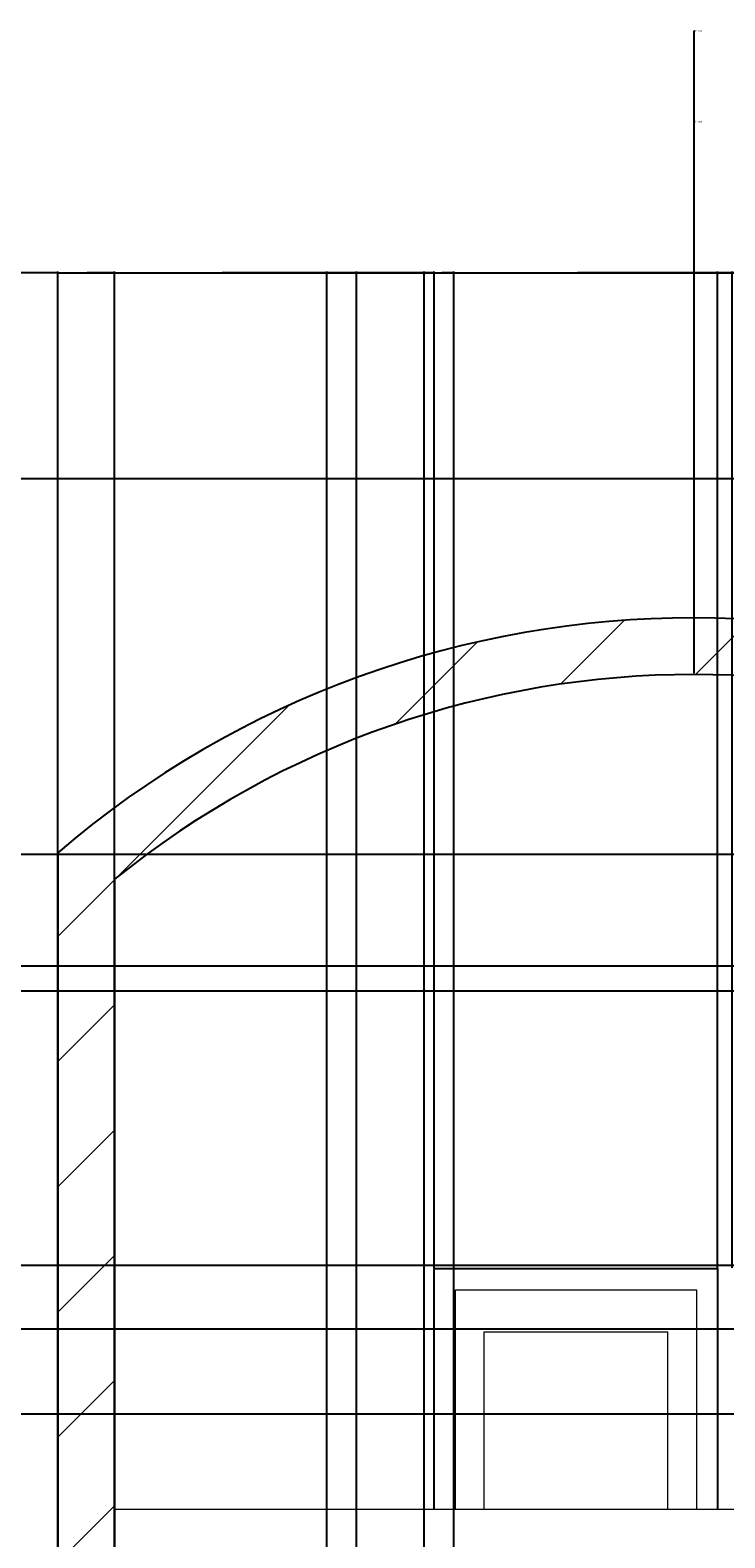
# Model space of a CAD drawing. Units: inches. Extents: x -14 to 375, y -86 to 549.
# Tile 11 of 12: x 130 to 228, y 336 to 549. Entities that reach past the tile are written whole.
import ezdxf

# ---------------------------------------------------------------- set-up
doc = ezdxf.new("R2010")
doc.units = ezdxf.units.IN
doc.header["$MEASUREMENT"] = 0
for name, color, linetype, lineweight in [('A-ANNO-DIMS', 2, 'Continuous', 18), ('A-DOOR', 3, 'Continuous', 18), ('A-ELEV', 7, 'Continuous', 25), ('A-ELEV-PATT', 8, 'Continuous', 13), ('A-ELEV-RAIL', 8, 'Continuous', 18)]:
    doc.layers.add(name, color=color, linetype=linetype, lineweight=lineweight)
doc.styles.get("Standard").update_dxf_attribs({"font": 'arial.ttf'})
doc.dimstyles.get("Standard").update_dxf_attribs({"dimtxt": 0.18, "dimasz": 0.18, "dimexe": 0.18, "dimexo": 0.0625, "dimgap": 0.09, "dimtad": 0, "dimtih": 1, "dimtoh": 1, "dimdec": 4, "dimzin": 0, "dimdsep": 46, "dimtxsty": 'Standard', "dimcen": 0.09, "dimadec": 0, "dimazin": 0, "dimtfac": 1, "dimtdec": 4, "dimtofl": 0, "dimtmove": 0, "dimatfit": 3, "dimfxl": 1, "dimtolj": 1, "dimtzin": 0, "dimarcsym": 0})

# ---------------------------------------------------------------- blocks, each defined once
blk = doc.blocks.new('*D7')
at = {"layer": 'A-ANNO-DIMS', "color": 0, "lineweight": -2, "transparency": 16777216}
for p, q in [((111.5, 433.03), (111.5, 515.24)), ((134.23, 433.23), (134.23, 515.24)), ((111.68, 515.06), (122.4, 515.06)), ((134.05, 515.06), (123.33, 515.06))]:
    blk.add_line(p, q, dxfattribs=at)
at = {"layer": 'A-ANNO-DIMS', "color": 0, "transparency": 16777216}
for points in [[(111.68, 515.09), (111.68, 515.03), (111.5, 515.06)], [(134.05, 515.09), (134.05, 515.03), (134.23, 515.06)]]:
    blk.add_solid(points, dxfattribs=at)
at = {"layer": 'Defpoints', "color": 0, "transparency": 16777216}
for p in [(134.23, 515.06), (111.5, 432.97), (134.23, 433.17)]:
    blk.add_point(p, dxfattribs=at)
at = {"layer": 'A-ANNO-DIMS', "color": 0, "transparency": 16777216, "insert": (122.87, 515.06), "char_height": 0.18, "attachment_point": 5}
blk.add_mtext('\\A1;22.735', dxfattribs=at)
blk = doc.blocks.new('*D8')
at = {"layer": 'A-ANNO-DIMS', "color": 0, "lineweight": -2, "transparency": 16777216}
for p, q in [((134.23, 433.23), (134.23, 515.24)), ((313.77, 433.23), (313.77, 515.24)), ((134.41, 515.06), (223.55, 515.06)), ((313.59, 515.06), (224.46, 515.06))]:
    blk.add_line(p, q, dxfattribs=at)
at = {"layer": 'A-ANNO-DIMS', "color": 0, "transparency": 16777216}
for points in [[(134.41, 515.09), (134.41, 515.03), (134.23, 515.06)], [(313.59, 515.09), (313.59, 515.03), (313.77, 515.06)]]:
    blk.add_solid(points, dxfattribs=at)
at = {"layer": 'Defpoints', "color": 0, "transparency": 16777216}
for p in [(313.77, 515.06), (134.23, 433.17), (313.77, 433.17)]:
    blk.add_point(p, dxfattribs=at)
at = {"layer": 'A-ANNO-DIMS', "color": 0, "transparency": 16777216, "insert": (224, 515.06), "char_height": 0.18, "attachment_point": 5}
blk.add_mtext('\\A1;179.54', dxfattribs=at)
blk = doc.blocks.new('*D17')
at = {"layer": 'A-ANNO-DIMS', "color": 0, "lineweight": -2, "transparency": 16777216}
for p, q in [((38.44, 432.97), (-13.88, 432.97)), ((-13.7, 432.79), (-13.7, 348.02)), ((-13.7, 262.89), (-13.7, 347.66)), ((134.17, 262.71), (-13.88, 262.71))]:
    blk.add_line(p, q, dxfattribs=at)
at = {"layer": 'A-ANNO-DIMS', "color": 0, "transparency": 16777216}
for points in [[(-13.73, 432.79), (-13.67, 432.79), (-13.7, 432.97)], [(-13.73, 262.89), (-13.67, 262.89), (-13.7, 262.71)]]:
    blk.add_solid(points, dxfattribs=at)
at = {"layer": 'Defpoints', "color": 0, "transparency": 16777216}
for p in [(-13.7, 432.97), (38.5, 432.97), (134.23, 262.71)]:
    blk.add_point(p, dxfattribs=at)
at = {"layer": 'A-ANNO-DIMS', "color": 0, "transparency": 16777216, "insert": (-13.7, 347.84), "char_height": 0.18, "attachment_point": 5}
blk.add_mtext('\\A1;170.26', dxfattribs=at)
blk = doc.blocks.new('*D36')
at = {"layer": 'A-ANNO-DIMS', "color": 0, "lineweight": -2, "transparency": 16777216}
for p, q in [((107.56, 353.96), (374.54, 353.96)), ((374.36, 353.78), (374.36, 327.93)), ((374.36, 301.72), (374.36, 327.57)), ((107.64, 301.54), (374.54, 301.54))]:
    blk.add_line(p, q, dxfattribs=at)
at = {"layer": 'A-ANNO-DIMS', "color": 0, "transparency": 16777216}
for points in [[(374.33, 353.78), (374.39, 353.78), (374.36, 353.96)], [(374.33, 301.72), (374.39, 301.72), (374.36, 301.54)]]:
    blk.add_solid(points, dxfattribs=at)
at = {"layer": 'Defpoints', "color": 0, "transparency": 16777216}
for p in [(107.5, 353.96), (374.36, 353.96), (107.58, 301.54)]:
    blk.add_point(p, dxfattribs=at)
at = {"layer": 'A-ANNO-DIMS', "color": 0, "transparency": 16777216, "insert": (374.36, 327.75), "char_height": 0.18, "attachment_point": 5}
blk.add_mtext('\\A1;52.42', dxfattribs=at)
blk = doc.blocks.new('*D37')
at = {"layer": 'A-ANNO-DIMS', "color": 0, "lineweight": -2, "transparency": 16777216}
for p, q in [((107.76, 365.96), (374.54, 365.96)), ((374.36, 365.78), (374.36, 360.14)), ((374.36, 354.14), (374.36, 359.78)), ((107.56, 353.96), (374.54, 353.96))]:
    blk.add_line(p, q, dxfattribs=at)
at = {"layer": 'A-ANNO-DIMS', "color": 0, "transparency": 16777216}
for points in [[(374.33, 365.78), (374.39, 365.78), (374.36, 365.96)], [(374.33, 354.14), (374.39, 354.14), (374.36, 353.96)]]:
    blk.add_solid(points, dxfattribs=at)
at = {"layer": 'Defpoints', "color": 0, "transparency": 16777216}
for p in [(107.7, 365.96), (374.36, 365.96), (107.5, 353.96)]:
    blk.add_point(p, dxfattribs=at)
at = {"layer": 'A-ANNO-DIMS', "color": 0, "transparency": 16777216, "insert": (374.36, 359.96), "char_height": 0.18, "attachment_point": 5}
blk.add_mtext('\\A1;12', dxfattribs=at)
blk = doc.blocks.new('*D38')
at = {"layer": 'A-ANNO-DIMS', "color": 0, "lineweight": -2, "transparency": 16777216}
for p, q in [((107.56, 374.96), (374.54, 374.96)), ((374.36, 374.78), (374.36, 370.64)), ((374.36, 366.14), (374.36, 370.28)), ((107.76, 365.96), (374.54, 365.96))]:
    blk.add_line(p, q, dxfattribs=at)
at = {"layer": 'A-ANNO-DIMS', "color": 0, "transparency": 16777216}
for points in [[(374.33, 374.78), (374.39, 374.78), (374.36, 374.96)], [(374.33, 366.14), (374.39, 366.14), (374.36, 365.96)]]:
    blk.add_solid(points, dxfattribs=at)
at = {"layer": 'Defpoints', "color": 0, "transparency": 16777216}
for p in [(107.5, 374.96), (374.36, 374.96), (107.7, 365.96)]:
    blk.add_point(p, dxfattribs=at)
at = {"layer": 'A-ANNO-DIMS', "color": 0, "transparency": 16777216, "insert": (374.36, 370.46), "char_height": 0.18, "attachment_point": 5}
blk.add_mtext('\\A1;9', dxfattribs=at)
blk = doc.blocks.new('*D39')
at = {"layer": 'A-ANNO-DIMS', "color": 0, "lineweight": -2, "transparency": 16777216}
for p, q in [((107.56, 413.68), (374.54, 413.68)), ((374.36, 413.5), (374.36, 394.5)), ((374.36, 375.14), (374.36, 394.14)), ((107.56, 374.96), (374.54, 374.96))]:
    blk.add_line(p, q, dxfattribs=at)
at = {"layer": 'A-ANNO-DIMS', "color": 0, "transparency": 16777216}
for points in [[(374.33, 413.5), (374.39, 413.5), (374.36, 413.68)], [(374.33, 375.14), (374.39, 375.14), (374.36, 374.96)]]:
    blk.add_solid(points, dxfattribs=at)
at = {"layer": 'Defpoints', "color": 0, "transparency": 16777216}
for p in [(107.5, 413.68), (374.36, 413.68), (107.5, 374.96)]:
    blk.add_point(p, dxfattribs=at)
at = {"layer": 'A-ANNO-DIMS', "color": 0, "transparency": 16777216, "insert": (374.36, 394.32), "char_height": 0.18, "attachment_point": 5}
blk.add_mtext('\\A1;38.72', dxfattribs=at)
blk = doc.blocks.new('*D40')
at = {"layer": 'A-ANNO-DIMS', "color": 0, "lineweight": -2, "transparency": 16777216}
for p, q in [((107.56, 417.18), (374.54, 417.18)), ((374.36, 417), (374.36, 415.61)), ((374.36, 413.86), (374.36, 415.25)), ((107.56, 413.68), (374.54, 413.68))]:
    blk.add_line(p, q, dxfattribs=at)
at = {"layer": 'A-ANNO-DIMS', "color": 0, "transparency": 16777216}
for points in [[(374.33, 417), (374.39, 417), (374.36, 417.18)], [(374.33, 413.86), (374.39, 413.86), (374.36, 413.68)]]:
    blk.add_solid(points, dxfattribs=at)
at = {"layer": 'Defpoints', "color": 0, "transparency": 16777216}
for p in [(107.5, 417.18), (374.36, 417.18), (107.5, 413.68)]:
    blk.add_point(p, dxfattribs=at)
at = {"layer": 'A-ANNO-DIMS', "color": 0, "transparency": 16777216, "insert": (374.36, 415.43), "char_height": 0.18, "attachment_point": 5}
blk.add_mtext('\\A1;3.501', dxfattribs=at)
blk = doc.blocks.new('*D41')
at = {"layer": 'A-ANNO-DIMS', "color": 0, "lineweight": -2, "transparency": 16777216}
for p, q in [((111.56, 432.97), (374.54, 432.97)), ((374.36, 432.79), (374.36, 425.26)), ((374.36, 417.36), (374.36, 424.89)), ((107.56, 417.18), (374.54, 417.18))]:
    blk.add_line(p, q, dxfattribs=at)
at = {"layer": 'A-ANNO-DIMS', "color": 0, "transparency": 16777216}
for points in [[(374.33, 432.79), (374.39, 432.79), (374.36, 432.97)], [(374.33, 417.36), (374.39, 417.36), (374.36, 417.18)]]:
    blk.add_solid(points, dxfattribs=at)
at = {"layer": 'Defpoints', "color": 0, "transparency": 16777216}
for p in [(111.5, 432.97), (374.36, 432.97), (107.5, 417.18)]:
    blk.add_point(p, dxfattribs=at)
at = {"layer": 'A-ANNO-DIMS', "color": 0, "transparency": 16777216, "insert": (374.36, 425.07), "char_height": 0.18, "attachment_point": 5}
blk.add_mtext('\\A1;15.786', dxfattribs=at)
blk = doc.blocks.new('*D53')
at = {"layer": 'A-ANNO-DIMS', "color": 0, "lineweight": -2, "transparency": 16777216}
for p, q in [((142.23, 429.48), (142.23, 515.24)), ((187.37, 374.55), (187.37, 515.24)), ((142.41, 515.06), (164.4, 515.06)), ((187.19, 515.06), (165.2, 515.06))]:
    blk.add_line(p, q, dxfattribs=at)
at = {"layer": 'A-ANNO-DIMS', "color": 0, "transparency": 16777216}
for points in [[(142.41, 515.09), (142.41, 515.03), (142.23, 515.06)], [(187.19, 515.09), (187.19, 515.03), (187.37, 515.06)]]:
    blk.add_solid(points, dxfattribs=at)
at = {"layer": 'Defpoints', "color": 0, "transparency": 16777216}
for p in [(187.37, 515.06), (142.23, 429.42), (187.37, 374.49)]:
    blk.add_point(p, dxfattribs=at)
at = {"layer": 'A-ANNO-DIMS', "color": 0, "transparency": 16777216, "insert": (164.8, 515.06), "char_height": 0.18, "attachment_point": 5}
blk.add_mtext('\\A1;45.13', dxfattribs=at)
blk = doc.blocks.new('*D54')
at = {"layer": 'A-ANNO-DIMS', "color": 0, "lineweight": -2, "transparency": 16777216}
for p, q in [((187.37, 374.55), (187.37, 515.24)), ((227.37, 374.55), (227.37, 515.24)), ((187.55, 515.06), (207.14, 515.06)), ((227.19, 515.06), (207.59, 515.06))]:
    blk.add_line(p, q, dxfattribs=at)
at = {"layer": 'A-ANNO-DIMS', "color": 0, "transparency": 16777216}
for points in [[(187.55, 515.09), (187.55, 515.03), (187.37, 515.06)], [(227.19, 515.09), (227.19, 515.03), (227.37, 515.06)]]:
    blk.add_solid(points, dxfattribs=at)
at = {"layer": 'Defpoints', "color": 0, "transparency": 16777216}
for p in [(227.37, 515.06), (187.37, 374.49), (227.37, 374.49)]:
    blk.add_point(p, dxfattribs=at)
at = {"layer": 'A-ANNO-DIMS', "color": 0, "transparency": 16777216, "insert": (207.37, 515.06), "char_height": 0.18, "attachment_point": 5}
blk.add_mtext('\\A1;40', dxfattribs=at)
blk = doc.blocks.new('*D55')
at = {"layer": 'A-ANNO-DIMS', "color": 0, "lineweight": -2, "transparency": 16777216}
for p, q in [((227.37, 374.55), (227.37, 515.24)), ((229.41, 374.55), (229.41, 515.24)), ((227.55, 515.06), (228.06, 515.06)), ((229.23, 515.06), (228.71, 515.06))]:
    blk.add_line(p, q, dxfattribs=at)
at = {"layer": 'A-ANNO-DIMS', "color": 0, "transparency": 16777216}
for points in [[(227.55, 515.09), (227.55, 515.03), (227.37, 515.06)], [(229.23, 515.09), (229.23, 515.03), (229.41, 515.06)]]:
    blk.add_solid(points, dxfattribs=at)
at = {"layer": 'Defpoints', "color": 0, "transparency": 16777216}
for p in [(229.41, 515.06), (227.37, 374.49), (229.41, 374.49)]:
    blk.add_point(p, dxfattribs=at)
at = {"layer": 'A-ANNO-DIMS', "color": 0, "transparency": 16777216, "insert": (228.39, 515.06), "char_height": 0.18, "attachment_point": 5}
blk.add_mtext('\\A1;2.04', dxfattribs=at)
blk = doc.blocks.new('*D99')
at = {"layer": 'A-ANNO-DIMS', "color": 0, "lineweight": -2, "transparency": 16777216}
for p, q in [((134.23, 6.02), (134.23, 515.24)), ((142.23, 6.02), (142.23, 515.24)), ((134.41, 515.06), (138.08, 515.06)), ((142.05, 515.06), (138.38, 515.06))]:
    blk.add_line(p, q, dxfattribs=at)
at = {"layer": 'A-ANNO-DIMS', "color": 0, "transparency": 16777216}
for points in [[(134.41, 515.09), (134.41, 515.03), (134.23, 515.06)], [(142.05, 515.09), (142.05, 515.03), (142.23, 515.06)]]:
    blk.add_solid(points, dxfattribs=at)
at = {"layer": 'Defpoints', "color": 0, "transparency": 16777216}
for p in [(142.23, 515.06), (134.23, 5.96), (142.23, 5.96)]:
    blk.add_point(p, dxfattribs=at)
at = {"layer": 'A-ANNO-DIMS', "color": 0, "transparency": 16777216, "insert": (138.23, 515.06), "char_height": 0.18, "attachment_point": 5}
blk.add_mtext('\\A1;8', dxfattribs=at)
blk = doc.blocks.new('*D100')
at = {"layer": 'A-ANNO-DIMS', "color": 0, "lineweight": -2, "transparency": 16777216}
for p, q in [((142.23, 6.02), (142.23, 515.24)), ((172.23, 6.02), (172.23, 515.24)), ((142.41, 515.06), (157.01, 515.06)), ((172.05, 515.06), (157.45, 515.06))]:
    blk.add_line(p, q, dxfattribs=at)
at = {"layer": 'A-ANNO-DIMS', "color": 0, "transparency": 16777216}
for points in [[(142.41, 515.09), (142.41, 515.03), (142.23, 515.06)], [(172.05, 515.09), (172.05, 515.03), (172.23, 515.06)]]:
    blk.add_solid(points, dxfattribs=at)
at = {"layer": 'Defpoints', "color": 0, "transparency": 16777216}
for p in [(172.23, 515.06), (142.23, 5.96), (172.23, 5.96)]:
    blk.add_point(p, dxfattribs=at)
at = {"layer": 'A-ANNO-DIMS', "color": 0, "transparency": 16777216, "insert": (157.23, 515.06), "char_height": 0.18, "attachment_point": 5}
blk.add_mtext('\\A1;30', dxfattribs=at)
blk = doc.blocks.new('*D101')
at = {"layer": 'A-ANNO-DIMS', "color": 0, "lineweight": -2, "transparency": 16777216}
for p, q in [((172.23, 6.02), (172.23, 515.24)), ((176.42, 6.02), (176.42, 515.24)), ((172.41, 515.06), (173.93, 515.06)), ((176.24, 515.06), (174.72, 515.06))]:
    blk.add_line(p, q, dxfattribs=at)
at = {"layer": 'A-ANNO-DIMS', "color": 0, "transparency": 16777216}
for points in [[(172.41, 515.09), (172.41, 515.03), (172.23, 515.06)], [(176.24, 515.09), (176.24, 515.03), (176.42, 515.06)]]:
    blk.add_solid(points, dxfattribs=at)
at = {"layer": 'Defpoints', "color": 0, "transparency": 16777216}
for p in [(176.42, 515.06), (172.23, 5.96), (176.42, 5.96)]:
    blk.add_point(p, dxfattribs=at)
at = {"layer": 'A-ANNO-DIMS', "color": 0, "transparency": 16777216, "insert": (174.32, 515.06), "char_height": 0.18, "attachment_point": 5}
blk.add_mtext('\\A1;4.186', dxfattribs=at)
blk = doc.blocks.new('*D102')
at = {"layer": 'A-ANNO-DIMS', "color": 0, "lineweight": -2, "transparency": 16777216}
for p, q in [((176.42, 6.02), (176.42, 515.24)), ((185.96, 6.02), (185.96, 515.24)), ((176.6, 515.06), (180.8, 515.06)), ((185.78, 515.06), (181.58, 515.06))]:
    blk.add_line(p, q, dxfattribs=at)
at = {"layer": 'A-ANNO-DIMS', "color": 0, "transparency": 16777216}
for points in [[(176.6, 515.09), (176.6, 515.03), (176.42, 515.06)], [(185.78, 515.09), (185.78, 515.03), (185.96, 515.06)]]:
    blk.add_solid(points, dxfattribs=at)
at = {"layer": 'Defpoints', "color": 0, "transparency": 16777216}
for p in [(185.96, 515.06), (176.42, 5.96), (185.96, 5.96)]:
    blk.add_point(p, dxfattribs=at)
at = {"layer": 'A-ANNO-DIMS', "color": 0, "transparency": 16777216, "insert": (181.19, 515.06), "char_height": 0.18, "attachment_point": 5}
blk.add_mtext('\\A1;9.545', dxfattribs=at)
blk = doc.blocks.new('*D103')
at = {"layer": 'A-ANNO-DIMS', "color": 0, "lineweight": -2, "transparency": 16777216}
for p, q in [((185.96, 6.02), (185.96, 515.24)), ((190.15, 6.02), (190.15, 515.24)), ((186.14, 515.06), (187.66, 515.06)), ((189.97, 515.06), (188.45, 515.06))]:
    blk.add_line(p, q, dxfattribs=at)
at = {"layer": 'A-ANNO-DIMS', "color": 0, "transparency": 16777216}
for points in [[(186.14, 515.09), (186.14, 515.03), (185.96, 515.06)], [(189.97, 515.09), (189.97, 515.03), (190.15, 515.06)]]:
    blk.add_solid(points, dxfattribs=at)
at = {"layer": 'Defpoints', "color": 0, "transparency": 16777216}
for p in [(190.15, 515.06), (185.96, 5.96), (190.15, 5.96)]:
    blk.add_point(p, dxfattribs=at)
at = {"layer": 'A-ANNO-DIMS', "color": 0, "transparency": 16777216, "insert": (188.06, 515.06), "char_height": 0.18, "attachment_point": 5}
blk.add_mtext('\\A1;4.186', dxfattribs=at)
blk = doc.blocks.new('*D104')
at = {"layer": 'A-ANNO-DIMS', "color": 0, "lineweight": -2, "transparency": 16777216}
for p, q in [((190.15, 6.02), (190.15, 515.24)), ((271, 6.02), (271, 515.24)), ((190.33, 515.06), (230.18, 515.06)), ((270.82, 515.06), (230.97, 515.06))]:
    blk.add_line(p, q, dxfattribs=at)
at = {"layer": 'A-ANNO-DIMS', "color": 0, "transparency": 16777216}
for points in [[(190.33, 515.09), (190.33, 515.03), (190.15, 515.06)], [(270.82, 515.09), (270.82, 515.03), (271, 515.06)]]:
    blk.add_solid(points, dxfattribs=at)
at = {"layer": 'Defpoints', "color": 0, "transparency": 16777216}
for p in [(271, 515.06), (190.15, 5.96), (271, 5.96)]:
    blk.add_point(p, dxfattribs=at)
at = {"layer": 'A-ANNO-DIMS', "color": 0, "transparency": 16777216, "insert": (230.57, 515.06), "char_height": 0.18, "attachment_point": 5}
blk.add_mtext('\\A1;80.85', dxfattribs=at)
blk = doc.blocks.new('*D133')
at = {"layer": 'A-ANNO-DIMS', "color": 0, "lineweight": -2, "transparency": 16777216}
for p, q in [((224.18, 549.18), (224, 549.18)), ((224, 549.18), (224, 466.51)), ((223.91, 328.25), (224.09, 328.25)), ((224, 328.16), (224, 328.34))]:
    blk.add_line(p, q, dxfattribs=at)
at = {"layer": 'A-ANNO-DIMS', "color": 0, "transparency": 16777216}
blk.add_solid([(223.97, 466.51), (224.03, 466.51), (224, 466.33)], dxfattribs=at)
at = {"layer": 'Defpoints', "color": 0, "transparency": 16777216}
for p in [(224, 466.33), (224, 328.25)]:
    blk.add_point(p, dxfattribs=at)
at = {"layer": 'A-ANNO-DIMS', "color": 0, "transparency": 16777216, "insert": (224.73, 549.18), "char_height": 0.18, "attachment_point": 5}
blk.add_mtext('\\A1;R138.08', dxfattribs=at)
blk = doc.blocks.new('*D134')
at = {"layer": 'A-ANNO-DIMS', "color": 0, "lineweight": -2, "transparency": 16777216}
for p, q in [((224.18, 536.38), (224, 536.38)), ((224, 536.38), (224, 458.51)), ((223.91, 328.25), (224.09, 328.25)), ((224, 328.16), (224, 328.34))]:
    blk.add_line(p, q, dxfattribs=at)
at = {"layer": 'A-ANNO-DIMS', "color": 0, "transparency": 16777216}
blk.add_solid([(223.97, 458.51), (224.03, 458.51), (224, 458.33)], dxfattribs=at)
at = {"layer": 'Defpoints', "color": 0, "transparency": 16777216}
for p in [(224, 458.33), (224, 328.25)]:
    blk.add_point(p, dxfattribs=at)
at = {"layer": 'A-ANNO-DIMS', "color": 0, "transparency": 16777216, "insert": (224.73, 536.38), "char_height": 0.18, "attachment_point": 5}
blk.add_mtext('\\A1;R130.08', dxfattribs=at)

msp = doc.modelspace()

# ---------------------------------------------------------------- hatches: boundary and pattern name
at = {"layer": 'A-ELEV-PATT'}
h = msp.add_hatch(dxfattribs=at)
h.set_pattern_fill('ANSI31', color=256, scale=100)
h.set_pattern_definition([(45, (-168.406, -22.703), (-8.83883, 8.83883), [])])
h.paths.add_polyline_path([(313.6281, 262.7071), (313.6281, 357.9589), (313.7701, 357.9589), (313.7701, 433.1717, 0.36940998), (134.2334, 433.1717), (134.2334, 365.9589), (134.2334, 262.7071)])
h.paths.add_polyline_path([(142.2334, 270.7071), (142.2334, 365.9589), (142.2334, 429.4208, -0.35358711), (305.7701, 429.4208), (305.7701, 365.9589), (305.6281, 365.9589), (305.6281, 270.7071)], flags=16)
h.paths.add_polyline_path([(134.2334, 187.8466), (134.2334, 117.9589), (313.7701, 117.9589), (313.7701, 187.8466, 0.62486768)])
h.paths.add_polyline_path([(305.7701, 185.9589), (305.7701, 125.9589), (142.2334, 125.9589), (142.2334, 185.9589, -0.61125102)], flags=16)
h.paths.add_polyline_path([(134.2334, 73.1717), (134.2334, 5.9589), (142.2334, 5.9589), (142.2334, 69.4208, -0.35358711), (305.7701, 69.4208), (305.7701, 5.9589), (313.7701, 5.9589), (313.7701, 73.1717, 0.36940998)])

# ---------------------------------------------------------------- linework, layer by layer
at = {"layer": 'A-DOOR'}
for points in [[(190.3657, 340.4421), (190.3657, 371.4627), (224.3657, 371.4627), (224.3657, 340.4421)], [(220.3657, 340.4421), (220.3657, 365.4627), (194.3657, 365.4627), (194.3657, 340.4421)]]:
    msp.add_lwpolyline(points, dxfattribs=at)
at = {"layer": 'A-ELEV'}
msp.add_line((301.4553, 485.9589), (59.2112, 485.9589), dxfattribs=at)
for points in [[(134.2334, 262.7071), (313.6281, 262.7071), (313.6281, 357.9589), (313.7701, 357.9589), (313.7701, 433.1717, 0.36940998), (134.2334, 433.1717), (134.2334, 365.9589)], [(142.2334, 270.7071), (305.6281, 270.7071), (305.6281, 365.9589), (305.7701, 365.9589), (305.7701, 429.4208, 0.35358711), (142.2334, 429.4208), (142.2334, 365.9589)]]:
    msp.add_lwpolyline(points, format="xyb", close=True, dxfattribs=at)
msp.add_lwpolyline([(187.3657, 340.4421), (187.3657, 374.4857), (227.3657, 374.4857), (227.3657, 340.4421)], dxfattribs=at)
at = {"layer": 'A-ELEV-RAIL'}
msp.add_line((305.6281, 340.4421), (142.2334, 340.4421), dxfattribs=at)

# ---------------------------------------------------------------- dimensions: what is measured, and where the dimension line sits
at = {"layer": 'A-ANNO-DIMS'}
for mpoint, picture, middle in [((224.002, 466.333), '*D133', (224.7321, 549.1828)), ((224.002, 458.333), '*D134', (224.7321, 536.3828))]:
    dim = msp.add_radius_dim(center=(224.0017, 328.25), mpoint=mpoint, dimstyle='Standard', override={"dimdec": 2, "dimlfac": 1, "dimrnd": 0, "dimzin": 0, "dimdsep": 46, "dimlunit": 2}, dxfattribs=at)
    dim.commit()
    dim.dimension.update_dxf_attribs({"geometry": picture, "text_midpoint": middle, "dimtype": 164})
for base, p1, p2, override, picture, middle in [((134.2334, 515.0589), (111.4987, 432.9679), (134.2334, 433.1717), {"dimdec": 3, "dimlfac": 1, "dimrnd": 0, "dimzin": 0, "dimdsep": 46, "dimlunit": 2}, '*D7', (122.866, 515.0589)), ((313.7701, 515.0589), (134.2334, 433.1717), (313.7701, 433.1717), {"dimdec": 2, "dimlfac": 1, "dimrnd": 0, "dimzin": 0, "dimdsep": 46, "dimlunit": 2}, '*D8', (224.0017, 515.0589)), ((142.2334, 515.0589), (134.2334, 5.9589), (142.2334, 5.9589), {"dimdec": 0, "dimlfac": 1, "dimrnd": 0, "dimzin": 0, "dimdsep": 46, "dimlunit": 2}, '*D99', (138.2334, 515.0589)), ((187.3657, 515.0589), (142.2334, 429.4208), (187.3657, 374.4857), {"dimdec": 2, "dimlfac": 1, "dimrnd": 0, "dimzin": 0, "dimdsep": 46, "dimlunit": 2}, '*D53', (164.7996, 515.0589)), ((172.2314, 515.0589), (142.2334, 5.9589), (172.2314, 5.9589), {"dimdec": 0, "dimlfac": 1, "dimrnd": 0, "dimzin": 0, "dimdsep": 46, "dimlunit": 2}, '*D100', (157.2324, 515.0589)), ((176.4171, 515.0589), (172.2314, 5.9589), (176.4171, 5.9589), {"dimdec": 3, "dimlfac": 1, "dimrnd": 0, "dimzin": 0, "dimdsep": 46, "dimlunit": 2}, '*D101', (174.3243, 515.0589)), ((185.9623, 515.0589), (176.4171, 5.9589), (185.9623, 5.9589), {"dimdec": 3, "dimlfac": 1, "dimrnd": 0, "dimzin": 0, "dimdsep": 46, "dimlunit": 2}, '*D102', (181.1897, 515.0589)), ((190.148, 515.0589), (185.9623, 5.9589), (190.148, 5.9589), {"dimdec": 3, "dimlfac": 1, "dimrnd": 0, "dimzin": 0, "dimdsep": 46, "dimlunit": 2}, '*D103', (188.0551, 515.0589)), ((227.3657, 515.0589), (187.3657, 374.4857), (227.3657, 374.4857), {"dimdec": 0, "dimlfac": 1, "dimrnd": 0, "dimzin": 0, "dimdsep": 46, "dimlunit": 2}, '*D54', (207.3657, 515.0589)), ((270.9993, 515.0589), (190.148, 5.9589), (270.9993, 5.9589), {"dimdec": 2, "dimlfac": 1, "dimrnd": 0, "dimzin": 0, "dimdsep": 46, "dimlunit": 2}, '*D104', (230.5736, 515.0589)), ((229.409, 515.0589), (227.3657, 374.4857), (229.409, 374.4857), {"dimdec": 2, "dimlfac": 1, "dimrnd": 0, "dimzin": 0, "dimdsep": 46, "dimlunit": 2}, '*D55', (228.3874, 515.0589))]:
    dim = msp.add_linear_dim(base=base, p1=p1, p2=p2, dimstyle='Standard', override=override, dxfattribs=at)
    dim.commit()
    dim.dimension.update_dxf_attribs({"geometry": picture, "text_midpoint": middle})
for base, p1, p2, override, picture, middle in [((-13.6982, 432.9679), (134.2334, 262.7071), (38.5033, 432.9679), {"dimdec": 2, "dimlfac": 1, "dimrnd": 0, "dimzin": 0, "dimdsep": 46, "dimlunit": 2}, '*D17', (-13.6982, 347.8375)), ((374.3647, 432.9679), (107.4987, 417.1817), (111.4987, 432.9679), {"dimdec": 3, "dimlfac": 1, "dimrnd": 0, "dimzin": 0, "dimdsep": 46, "dimlunit": 2}, '*D41', (374.3647, 425.0748)), ((374.3647, 417.1817), (107.4987, 413.6806), (107.4987, 417.1817), {"dimdec": 3, "dimlfac": 1, "dimrnd": 0, "dimzin": 0, "dimdsep": 46, "dimlunit": 2}, '*D40', (374.3647, 415.4312)), ((374.3647, 413.6806), (107.4987, 374.9589), (107.4987, 413.6806), {"dimdec": 2, "dimlfac": 1, "dimrnd": 0, "dimzin": 0, "dimdsep": 46, "dimlunit": 2}, '*D39', (374.3647, 394.3198)), ((374.3647, 374.9589), (107.7019, 365.9589), (107.4987, 374.9589), {"dimdec": 0, "dimlfac": 1, "dimrnd": 0, "dimzin": 0, "dimdsep": 46, "dimlunit": 2}, '*D38', (374.3647, 370.4589)), ((374.3647, 365.9589), (107.4987, 353.9589), (107.7019, 365.9589), {"dimdec": 0, "dimlfac": 1, "dimrnd": 0, "dimzin": 0, "dimdsep": 46, "dimlunit": 2}, '*D37', (374.3647, 359.9589)), ((374.3647, 353.9589), (107.5784, 301.5363), (107.4987, 353.9589), {"dimdec": 2, "dimlfac": 1, "dimrnd": 0, "dimzin": 0, "dimdsep": 46, "dimlunit": 2}, '*D36', (374.3647, 327.7476))]:
    dim = msp.add_linear_dim(base=base, p1=p1, p2=p2, angle=90, dimstyle='Standard', override=override, dxfattribs=at)
    dim.commit()
    dim.dimension.update_dxf_attribs({"geometry": picture, "text_midpoint": middle})

doc.saveas('drawing.dxf')
